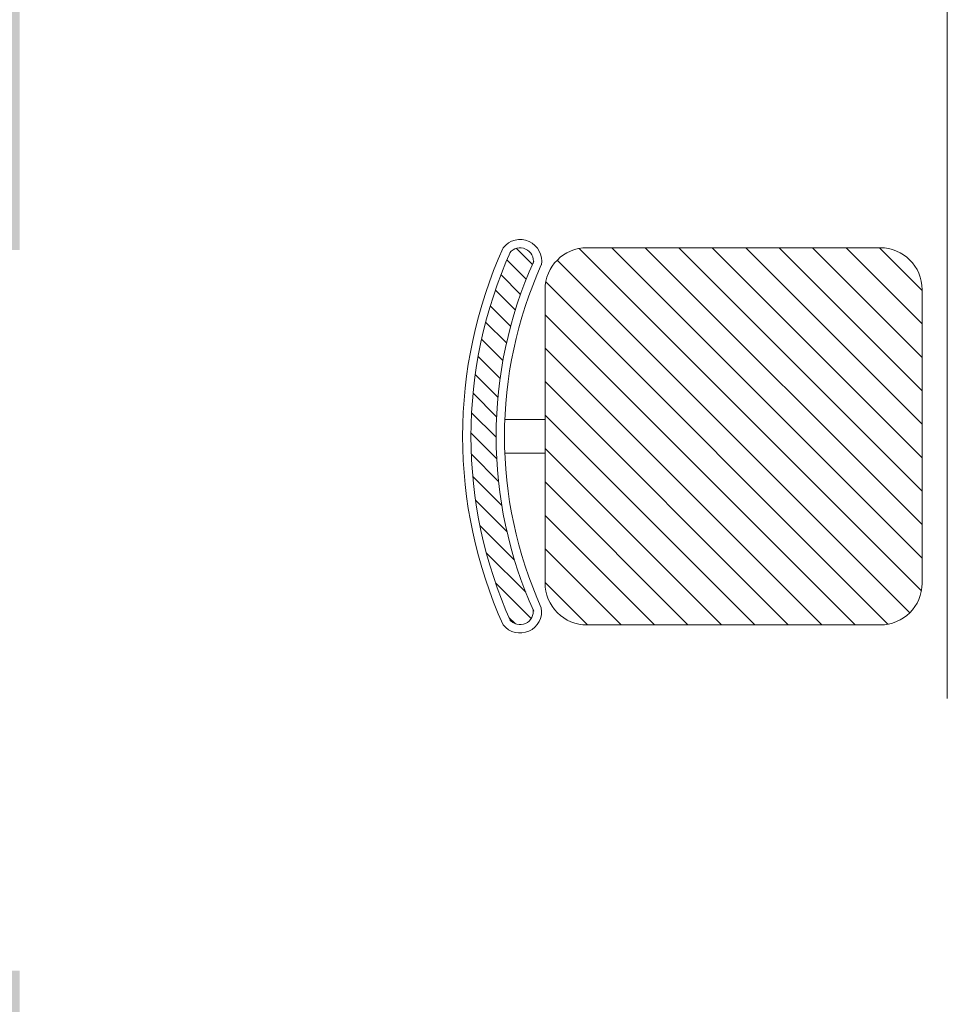
# Model space of a CAD drawing. Units: inches. Extents: x 375 to 1122, y 27 to 1069.
# Tile 84 of 155: x 667 to 705, y 846 to 887. Entities that reach past the tile are written whole.
import ezdxf

# ---------------------------------------------------------------- set-up
doc = ezdxf.new("R2010")
doc.units = ezdxf.units.IN
for name, color, linetype, lineweight in [('A-ANNO-DIMS', 2, 'Continuous', 18), ('A-WALL-PATT', 252, 'Continuous', 13), ('Furniture', 30, 'Continuous', 18)]:
    doc.layers.add(name, color=color, linetype=linetype, lineweight=lineweight)
doc.styles.get("Standard").update_dxf_attribs({"font": 'arial.ttf'})
doc.dimstyles.new('ISO-25', dxfattribs={"dimtxt": 12, "dimasz": 2.5, "dimexe": 1.5, "dimexo": 1.5, "dimtad": 1, "dimdec": 1, "dimlunit": 3, "dimtxsty": 'Standard', "dimblk": 'ARCHTICK', "dimcen": 2.5, "dimadec": 0, "dimazin": 0, "dimtfac": 1, "dimtdec": 1, "dimtmove": 0, "dimatfit": 3, "dimfxl": 1.5, "dimfxlon": 1, "dimarcsym": 0})

# ---------------------------------------------------------------- blocks, each defined once
blk = doc.blocks.new('A$C403C54AD')
for p, q in [((0.8357, 0.5048, -0.0006), (1.9992, 0.5048, -0.0006)), ((1.8792, 0.4785, -0.0006), (1.5738, 0.4785, -0.0006)), ((1.5302, 0.4349, -0.0006), (1.5302, 0.304, -0.0006)), ((1.9228, 0.1295, -0.0006), (1.9228, 0.4349, -0.0006)), ((1.5302, 0.304, -0.0006), (1.5302, 0.1295, -0.0006)), ((1.5738, 0.0859, -0.0006), (1.8792, 0.0859, -0.0006)), ((1.7091, 0.0859, -0.0006), (1.7091, 0.0436, -0.0006)), ((1.744, 0.0859, -0.0006), (1.744, 0.0436, -0.0006))]:
    blk.add_line(p, q)
at = {"ltscale": 0.05}
for p, q in [((1.8532, 0.4785, -0.0006), (1.5302, 0.1555, -0.0006)), ((1.8184, 0.4785, -0.0006), (1.5302, 0.1903, -0.0006)), ((1.7836, 0.4785, -0.0006), (1.5302, 0.2252, -0.0006)), ((1.7487, 0.4785, -0.0006), (1.5302, 0.26, -0.0006)), ((1.7139, 0.4785, -0.0006), (1.5302, 0.2948, -0.0006)), ((1.6791, 0.4785, -0.0006), (1.5302, 0.3296, -0.0006)), ((1.6443, 0.4785, -0.0006), (1.5302, 0.3645, -0.0006)), ((1.6094, 0.4785, -0.0006), (1.5302, 0.3993, -0.0006)), ((1.5746, 0.4785, -0.0006), (1.5302, 0.4341, -0.0006)), ((1.8873, 0.4778, -0.0006), (1.5309, 0.1214, -0.0006)), ((1.9101, 0.4658, -0.0006), (1.543, 0.0986, -0.0006)), ((1.9221, 0.4429, -0.0006), (1.5658, 0.0866, -0.0006)), ((1.9228, 0.4089, -0.0006), (1.5999, 0.0859, -0.0006)), ((1.9228, 0.374, -0.0006), (1.6347, 0.0859, -0.0006)), ((1.9228, 0.3392, -0.0006), (1.6695, 0.0859, -0.0006)), ((1.9228, 0.3044, -0.0006), (1.7043, 0.0859, -0.0006)), ((1.9228, 0.2695, -0.0006), (1.7392, 0.0859, -0.0006)), ((1.9228, 0.2347, -0.0006), (1.774, 0.0859, -0.0006)), ((1.9228, 0.1999, -0.0006), (1.8088, 0.0859, -0.0006)), ((1.9228, 0.1651, -0.0006), (1.8437, 0.0859, -0.0006)), ((1.9228, 0.1302, -0.0006), (1.8785, 0.0859, -0.0006)), ((1.5475, 0.0727, -0.0006), (1.5309, 0.0561, -0.0006)), ((1.5629, 0.0663, -0.0006), (1.5428, 0.0462, -0.0006)), ((1.8888, 0.0658, -0.0006), (1.8478, 0.0247, -0.0006)), ((1.9162, 0.0714, -0.0006), (1.8791, 0.0343, -0.0006)), ((1.5787, 0.0603, -0.0006), (1.5583, 0.04, -0.0006)), ((1.595, 0.0549, -0.0006), (1.5743, 0.0341, -0.0006)), ((1.8554, 0.0541, -0.0006), (1.8193, 0.018, -0.0006)), ((1.9217, 0.0551, -0.0006), (1.9149, 0.0482, -0.0006)), ((1.6119, 0.05, -0.0006), (1.5907, 0.0288, -0.0006)), ((1.6293, 0.0457, -0.0006), (1.6077, 0.024, -0.0006)), ((1.6474, 0.042, -0.0006), (1.6252, 0.0198, -0.0006)), ((1.8257, 0.0462, -0.0006), (1.793, 0.0135, -0.0006)), ((1.6662, 0.039, -0.0006), (1.6433, 0.0162, -0.0006)), ((1.6857, 0.0368, -0.0006), (1.6621, 0.0132, -0.0006)), ((1.7061, 0.0354, -0.0006), (1.6816, 0.0109, -0.0006)), ((1.7274, 0.0349, -0.0006), (1.7019, 0.0094, -0.0006)), ((1.7498, 0.0355, -0.0006), (1.723, 0.0087, -0.0006)), ((1.7734, 0.0374, -0.0006), (1.7451, 0.0091, -0.0006)), ((1.7986, 0.0408, -0.0006), (1.7684, 0.0106, -0.0006))]:
    blk.add_line(p, q, dxfattribs=at)
for centre, radius, start, end in [((1.5738, 0.4349, -0.0006), 0.0436, 90, 180), ((1.8792, 0.4349, -0.0006), 0.0436, 0, 90), ((1.5738, 0.1295, -0.0006), 0.0436, 180, 270), ((1.8792, 0.1295, -0.0006), 0.0436, 270, 0), ((1.5441, 0.0599, -0.0006), 0.0225, 79.7658, 231.6694), ((1.7265, 0.4774, -0.0006), 0.4338, 245.7176, 294.2824), ((1.9087, 0.0598, -0.0006), 0.0225, 308.8964, 99.6684), ((1.5441, 0.0599, -0.0006), 0.0138, 79.7658, 231.6694), ((1.7265, 0.4774, -0.0006), 0.4425, 245.7176, 294.2824), ((1.9087, 0.0598, -0.0006), 0.0138, 308.8964, 99.6684), ((1.7265, 0.4774, -0.0006), 0.4774, 245.7176, 294.2824), ((1.7265, 0.4774, -0.0006), 0.4687, 245.7176, 294.2824)]:
    blk.add_arc(centre, radius, start, end)
blk = doc.blocks.new('_ArchTick')
at = {"color": 0, "linetype": 'ByBlock', "const_width": 0.15}
blk.add_lwpolyline([(-0.5, -0.5), (0.5, 0.5)], dxfattribs=at)
blk = doc.blocks.new('*D58')
at = {"layer": 'A-ANNO-DIMS', "color": 0, "lineweight": -2, "transparency": 16777216}
for p, q in [((656.912, 835.528), (656.912, 940.287)), ((655.412, 835.528), (658.412, 835.528)), ((656.912, 750.836), (656.912, 835.528)), ((655.412, 750.836), (658.412, 750.836))]:
    blk.add_line(p, q, dxfattribs=at)
at = {"layer": 'Defpoints', "color": 0, "transparency": 16777216}
for p in [(638.071, 835.528), (656.912, 835.528), (638.071, 750.836)]:
    blk.add_point(p, dxfattribs=at)
at = {"layer": 'A-ANNO-DIMS', "color": 0, "lineweight": -2, "transparency": 16777216, "xscale": 2.5, "yscale": 2.5, "zscale": 2.5}
for p, rotation in [((656.912, 835.528), 90), ((656.912, 750.836), 270)]:
    blk.add_blockref('_ArchTick', p, dxfattribs=dict(at, rotation=rotation))
at = {"layer": 'A-ANNO-DIMS', "color": 0, "transparency": 16777216, "insert": (650.082, 889.157), "char_height": 12, "attachment_point": 5, "rotation": 90}
blk.add_mtext('7\'-0 1/2" TYP.', dxfattribs=at)
blk = doc.blocks.new('*D85')
at = {"layer": 'A-ANNO-DIMS', "color": 0, "lineweight": -2, "transparency": 16777216}
for p, q in [((401.507, 868.528), (398.507, 868.528)), ((400.007, 814.528), (400.007, 868.528)), ((401.507, 814.528), (398.507, 814.528))]:
    blk.add_line(p, q, dxfattribs=at)
at = {"layer": 'Defpoints', "color": 0, "transparency": 16777216}
for p in [(400.007, 868.528), (845.007, 868.528), (845.007, 814.528)]:
    blk.add_point(p, dxfattribs=at)
at = {"layer": 'A-ANNO-DIMS', "color": 0, "lineweight": -2, "transparency": 16777216, "xscale": 2.5, "yscale": 2.5, "zscale": 2.5}
for p, rotation in [((400.007, 868.528), 90), ((400.007, 814.528), 270)]:
    blk.add_blockref('_ArchTick', p, dxfattribs=dict(at, rotation=rotation))
at = {"layer": 'A-ANNO-DIMS', "color": 0, "transparency": 16777216, "insert": (393.255, 841.528), "char_height": 12, "attachment_point": 5, "rotation": 90}
blk.add_mtext('4\'-6"', dxfattribs=at)

msp = doc.modelspace()

# ---------------------------------------------------------------- hatches: boundary and pattern name
at = {"layer": 'A-WALL-PATT'}
h = msp.add_hatch(color=256, dxfattribs=at)
h.dxf.hatch_style = 1
h.paths.add_polyline_path([(962.007, 388.528), (989.007, 388.528), (989.007, 394.528), (962.007, 394.528), (932.007, 394.528), (932.007, 397.528), (923.007, 397.528), (923.007, 394.528), (842.007, 394.528), (842.007, 334.528), (839.507, 334.528), (839.507, 328.528), (854.007, 328.528), (854.007, 334.528), (848.007, 334.528), (848.007, 388.528), (953.007, 388.528), (953.007, 356.081), (962.007, 356.081), (962.007, 358.554), (989.007, 358.554), (989.007, 364.554), (962.007, 364.554)])
h.paths.add_polyline_path([(989.007, 502.528), (932.007, 502.528), (932.007, 583.528), (932.007, 593.528), (923.007, 593.528), (923.007, 583.528), (854.007, 583.528), (854.007, 556.528), (863.007, 556.528), (863.007, 574.528), (923.007, 574.528), (923.007, 502.528), (863.007, 502.528), (863.007, 520.528), (854.007, 520.528), (854.007, 502.528), (773.007, 502.528), (773.007, 493.528), (788.007, 493.528), (788.007, 402.028), (722.007, 402.028), (722.007, 373.528), (728.007, 373.528), (728.007, 396.028), (788.007, 396.028), (788.007, 373.528), (794.007, 373.528), (794.007, 430.528), (814.007, 430.528), (814.007, 436.528), (794.007, 436.528), (794.007, 493.528), (923.007, 493.528), (923.007, 487.528), (932.007, 487.528), (932.007, 493.528), (983.007, 493.528), (983.007, 473.528), (989.007, 473.528)])
h.paths.add_polyline_path([(797.007, 325.528), (805.007, 325.528), (805.007, 328.528), (807.507, 328.528), (807.507, 334.528), (791.007, 334.528), (791.007, 226.528), (770.757, 226.528), (770.757, 217.528), (791.007, 217.528), (791.007, 187.528), (855.007, 187.528), (855.007, 196.528), (797.007, 196.528)])
h.paths.add_polyline_path([(989.007, 238.528), (962.007, 238.528), (962.007, 256.424), (953.007, 256.424), (953.007, 229.528), (980.007, 229.528), (980.007, 196.528), (915.007, 196.528), (915.007, 187.528), (989.007, 187.528)])
h.paths.add_polyline_path([(962.007, 334.528), (884.007, 334.528), (884.007, 328.528), (918.007, 328.528), (918.007, 325.528), (932.007, 325.528), (932.007, 328.528), (953.007, 328.528), (953.007, 304.424), (962.007, 304.424)])
h.paths.add_polyline_path([(606.507, 283.528), (609.507, 283.528), (609.507, 289.528), (600.507, 289.528), (600.507, 196.528), (578.507, 196.528), (578.507, 187.528), (606.507, 187.528), (606.507, 196.528)])
h.paths.add_polyline_path([(666.507, 292.528), (660.507, 292.528), (660.507, 289.528), (633.507, 289.528), (633.507, 283.528), (660.507, 283.528), (660.507, 196.528), (628.007, 196.528), (628.007, 187.528), (630.534, 187.528), (630.534, 160.528), (636.534, 160.528), (636.534, 187.528), (660.507, 187.528), (660.507, 160.528), (666.507, 160.528), (666.507, 217.528), (686.757, 217.528), (686.757, 226.528), (666.507, 226.528)])
h.paths.add_polyline_path([(480.507, 256.424), (471.507, 256.424), (471.507, 238.528), (444.507, 238.528), (444.507, 187.528), (518.507, 187.528), (518.507, 196.528), (453.507, 196.528), (453.507, 229.528), (480.507, 229.528)])
h.paths.add_polyline_path([(480.507, 328.528), (652.507, 328.528), (652.507, 325.528), (660.507, 325.528), (660.507, 322.528), (666.507, 322.528), (666.507, 334.528), (507.507, 334.528), (507.507, 360.528), (498.507, 360.528), (498.507, 334.528), (471.507, 334.528), (471.507, 304.424), (480.507, 304.424)])
h.paths.add_polyline_path([(507.507, 484.528), (498.507, 484.528), (498.507, 444.528), (507.507, 444.528), (507.507, 454.528), (621.507, 454.528), (621.507, 460.528), (507.507, 460.528)])
h.paths.add_polyline_path([(672.507, 604.528), (683.257, 604.528), (683.257, 613.528), (669.507, 613.528), (669.507, 649.528), (663.507, 649.528), (663.507, 589.528), (507.507, 589.528), (507.507, 613.528), (498.507, 613.528), (498.507, 556.528), (507.507, 556.528), (507.507, 580.528), (663.507, 580.528), (663.507, 520.528), (669.507, 520.528), (669.507, 556.528), (683.257, 556.528), (683.257, 565.528), (672.507, 565.528)])
h.paths.add_polyline_path([(731.007, 667.528), (734.007, 667.528), (734.007, 676.528), (728.007, 676.528), (728.007, 715.528), (657.507, 715.528), (657.507, 709.528), (663.507, 709.528), (663.507, 673.528), (669.507, 673.528), (669.507, 709.528), (722.007, 709.528), (722.007, 613.528), (704.757, 613.528), (704.757, 604.528), (722.007, 604.528), (722.007, 565.528), (704.757, 565.528), (704.757, 556.528), (722.007, 556.528), (722.007, 502.528), (722.007, 460.528), (669.507, 460.528), (669.507, 496.528), (663.507, 496.528), (663.507, 460.528), (657.507, 460.528), (657.507, 454.528), (728.007, 454.528), (728.007, 493.528), (734.007, 493.528), (734.007, 502.528), (731.007, 502.528)])
h.paths.add_polyline_path([(986.007, 718.528), (959.007, 718.528), (959.007, 727.528), (950.007, 727.528), (950.007, 709.528), (977.007, 709.528), (977.007, 676.528), (794.007, 676.528), (794.007, 805.528), (802.007, 805.528), (802.007, 808.528), (804.507, 808.528), (804.507, 814.528), (788.007, 814.528), (788.007, 774.028), (728.007, 774.028), (728.007, 796.528), (722.007, 796.528), (722.007, 768.028), (788.007, 768.028), (788.007, 676.528), (773.007, 676.528), (773.007, 667.528), (923.007, 667.528), (923.007, 657.528), (932.007, 657.528), (932.007, 667.528), (986.007, 667.528)])
h.paths.add_polyline_path([(621.507, 715.528), (507.507, 715.528), (507.507, 733.528), (498.507, 733.528), (498.507, 715.528), (498.507, 685.528), (507.507, 685.528), (507.507, 709.528), (621.507, 709.528)])
h.paths.add_polyline_path([(666.507, 847.028), (660.507, 847.028), (660.507, 844.528), (652.507, 844.528), (652.507, 841.528), (480.507, 841.528), (480.507, 859.528), (471.507, 859.528), (471.507, 835.528), (498.507, 835.528), (498.507, 817.528), (507.507, 817.528), (507.507, 835.528), (666.507, 835.528)])
h.paths.add_polyline_path([(480.507, 940.528), (453.507, 940.528), (453.507, 973.528), (518.507, 973.528), (518.507, 982.528), (444.507, 982.528), (444.507, 931.528), (471.507, 931.528), (471.507, 907.528), (480.507, 907.528)])
h.paths.add_polyline_path([(606.507, 982.528), (578.507, 982.528), (578.507, 973.528), (600.507, 973.528), (600.507, 880.528), (609.507, 880.528), (609.507, 886.528), (606.507, 886.528)])
h.paths.add_polyline_path([(666.507, 943.528), (686.757, 943.528), (686.757, 952.528), (666.507, 952.528), (666.507, 1009.528), (660.507, 1009.528), (660.507, 982.528), (636.534, 982.528), (636.534, 1009.528), (630.534, 1009.528), (630.534, 982.528), (628.007, 982.528), (628.007, 973.528), (660.507, 973.528), (660.507, 886.528), (633.507, 886.528), (633.507, 880.528), (660.507, 880.528), (660.507, 877.028), (666.507, 877.028)])
h.paths.add_polyline_path([(986.007, 874.528), (932.007, 874.528), (932.007, 877.528), (923.007, 877.528), (923.007, 874.528), (788.007, 874.528), (788.007, 868.528), (788.007, 844.528), (794.007, 844.528), (794.007, 868.528), (839.007, 868.528), (839.007, 814.528), (836.507, 814.528), (836.507, 808.528), (851.007, 808.528), (851.007, 814.528), (845.007, 814.528), (845.007, 868.528), (986.007, 868.528)])
h.paths.add_polyline_path([(959.007, 838.554), (986.007, 838.554), (986.007, 844.554), (959.007, 844.554), (959.007, 847.028), (950.007, 847.028), (950.007, 814.528), (881.007, 814.528), (881.007, 808.528), (918.007, 808.528), (918.007, 805.528), (932.007, 805.528), (932.007, 808.528), (950.007, 808.528), (950.007, 793.528), (959.007, 793.528)])
h.paths.add_polyline_path([(986.007, 982.528), (899.007, 982.528), (899.007, 973.528), (923.007, 973.528), (923.007, 967.528), (932.007, 967.528), (932.007, 973.528), (980.007, 973.528), (980.007, 953.528), (986.007, 953.528)])
h.paths.add_polyline_path([(851.007, 982.528), (788.007, 982.528), (788.007, 952.528), (770.757, 952.528), (770.757, 943.528), (788.007, 943.528), (788.007, 910.528), (814.007, 910.528), (814.007, 916.528), (794.007, 916.528), (794.007, 973.528), (851.007, 973.528)])

# ---------------------------------------------------------------- block references
at = {"layer": 'Furniture', "xscale": 39.9918517141215, "yscale": 39.9918517141215, "zscale": 39.9918517141215, "rotation": 270}
msp.add_blockref('A$C403C54AD', (684.955, 938.316, 0.024), dxfattribs=at)

# ---------------------------------------------------------------- dimensions: what is measured, and where the dimension line sits
at = {"layer": 'A-ANNO-DIMS'}
dim = msp.add_linear_dim(base=(656.912, 835.528), p1=(638.071, 750.836), p2=(638.071, 835.528), angle=90, text='<> TYP.', dimstyle='ISO-25', override={"dimdec": 1, "dimlfac": 1, "dimrnd": 0, "dimzin": 1, "dimdsep": 46, "dimlunit": 4, "dimfrac": 2}, dxfattribs=at)
dim.commit()
dim.dimension.update_dxf_attribs({"geometry": '*D58', "text_midpoint": (650.082, 889.157)})
dim = msp.add_linear_dim(base=(400.007, 868.528), p1=(845.007, 814.528), p2=(845.007, 868.528), angle=90, dimstyle='ISO-25', override={"dimdec": 1, "dimlfac": 1, "dimrnd": 0, "dimzin": 1, "dimdsep": 46, "dimlunit": 4, "dimfrac": 2}, dxfattribs=at)
dim.commit()
dim.dimension.update_dxf_attribs({"geometry": '*D85', "text_midpoint": (393.255, 841.528)})

doc.saveas('drawing.dxf')
